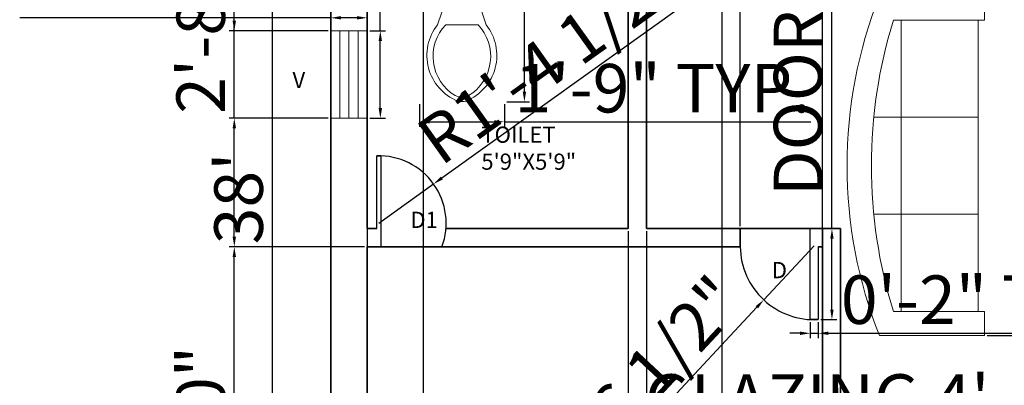
# Model space of a CAD drawing. Units: inches. Extents: x 2691 to 3133, y 1294 to 1993.
# Tile 2 of 7: x 2691 to 2935, y 1606 to 1696. Entities that reach past the tile are written whole.
import ezdxf

# ---------------------------------------------------------------- set-up
doc = ezdxf.new("R2010")
doc.units = ezdxf.units.IN
for name, color, linetype, lineweight in [('A-ANNO-DIMS', 2, 'Continuous', 18), ('A-ANNO-TEXT', 7, 'Continuous', 18), ('A-AREA-IDEN', 7, 'Continuous', 25), ('A-DOOR', 3, 'Continuous', 25), ('A-FLOR-FIXT', 9, 'Continuous', 18), ('A-FURN', 8, 'Continuous', 18), ('A-GLAZ', 4, 'Continuous', 18), ('A-WALL', 7, 'Continuous', 35)]:
    doc.layers.add(name, color=color, linetype=linetype, lineweight=lineweight)
doc.styles.get("Standard").update_dxf_attribs({"font": 'arial.ttf'})
doc.dimstyles.new('ISO-25', dxfattribs={"dimtxt": 12, "dimasz": 2.5, "dimexe": 1.25, "dimexo": 0.625, "dimtad": 1, "dimdec": 1, "dimlunit": 3, "dimtxsty": 'Standard', "dimcen": 2.5, "dimadec": 0, "dimazin": 0, "dimtfac": 1, "dimtdec": 1, "dimtmove": 0, "dimatfit": 3, "dimfxl": 1, "dimarcsym": 0})

# ---------------------------------------------------------------- blocks, each defined once
blk = doc.blocks.new('Sofa - Roundback 7 ft.')
for p, q in [((-12.00002, -32.4421), (-12.00003, -6.5971)), ((11.99997, -32.4421), (11.99998, -6.5971)), ((-36.000027, -34), (-36.000027, -11.4696)), ((35.99998, -34), (35.99998, -11.4696)), ((-35.999844, -13.3819), (35.9998, -13.3819)), ((-36.000027, -32.4421), (35.99998, -32.4421))]:
    blk.add_line(p, q)
for points in [[(-36.000027, -34), (-42.000027, -34), (-42.000027, -8)], [(41.99998, -8), (41.99998, -34), (35.99998, -34)]]:
    blk.add_lwpolyline(points)
for centre, radius, start, end in [((0, -114.25), 114.25, 68.43141, 111.5686), ((-0.00001, -127.1968), 121.1968, 72.72033, 107.2797)]:
    blk.add_arc(centre, radius, start, end)
blk = doc.blocks.new('Window - Wood Frame 36 in. Wide plan')
for p, q in [((0, 6), (0, 0)), ((36, 6), (36, 0)), ((0, 4.5), (36, 4.5)), ((0, 3), (36, 3)), ((0, 1.5), (36, 1.5))]:
    blk.add_line(p, q)
blk = doc.blocks.new('Toilet - top')
for p, q in [((9.5, -6), (9.5, -2)), ((-10, -8.5), (-8, -8.5)), ((-10, -9.5), (-10, -8.5)), ((-7, -9.5), (-10, -9.5)), ((-8, -8.5), (-8, -8)), ((-7, -8), (-7, -9.5)), ((-4, -8), (-6, -14)), ((4, -8), (6, -14)), ((4, -14), (-4, -14))]:
    blk.add_line(p, q)
blk.add_lwpolyline([(10.5, -8), (10.5, 0), (-10.5, 0), (-10.5, -8)], close=True)
for points in [[(-9.5, -2), (-9.5, -6)], [(8.5, -1), (-8.5, -1)], [(-8.5, -7), (8.5, -7)]]:
    blk.add_lwpolyline(points)
for centre, radius, start, end in [((-8.62, -1.88), 0.884, 81.8699, 188.1301), ((8.62, -1.88), 0.884, 351.8699, 98.1301), ((-8.62, -6.12), 0.884, 171.8699, 278.1301), ((8.62, -6.12), 0.884, 261.8699, 8.1301), ((3.52, -21.58), 12.17, 141.4691, 247.9714), ((4.2, -21.82), 11.33, 136.3677, 238.9468), ((-3.52, -21.58), 12.17, 292.0284, 38.5307), ((-4.2, -21.82), 11.33, 301.053, 43.6321), ((0, -27.88), 4, 245.7318, 294.2682), ((0, -29), 4, 254.8605, 285.1395)]:
    blk.add_arc(centre, radius, start, end)
blk = doc.blocks.new('*D11')
at = {"layer": 'A-ANNO-DIMS', "color": 0, "lineweight": -2, "transparency": 16777216}
for p, q in [((2767.62, 1880.05), (2752.52, 1880.05)), ((2753.77, 1877.55), (2753.77, 1426.55)), ((2767.62, 1424.05), (2752.52, 1424.05))]:
    blk.add_line(p, q, dxfattribs=at)
at = {"layer": 'A-ANNO-DIMS', "color": 0, "transparency": 16777216}
for points in [[(2753.35, 1877.55), (2754.18, 1877.55), (2753.77, 1880.05)], [(2753.35, 1426.55), (2754.18, 1426.55), (2753.77, 1424.05)]]:
    blk.add_solid(points, dxfattribs=at)
at = {"layer": 'Defpoints', "color": 0, "transparency": 16777216}
for p in [(2768.25, 1880.05), (2753.77, 1424.05), (2768.25, 1424.05)]:
    blk.add_point(p, dxfattribs=at)
at = {"layer": 'A-ANNO-DIMS', "color": 0, "transparency": 16777216, "insert": (2747.01, 1652.05), "char_height": 12, "attachment_point": 5, "rotation": 90}
blk.add_mtext("38'", dxfattribs=at)
blk = doc.blocks.new('DOOR-LEAF-THIN')
for p, q in [((18, 1), (0, 1)), ((0, 1), (0, 0)), ((0, 0), (22.5, 0))]:
    blk.add_line(p, q)
blk = doc.blocks.new('DOOR-LEAF-WIDE')
for p, q in [((0, 0), (0, 22.5)), ((2, 18), (2, 0)), ((2, 0), (0, 0))]:
    blk.add_line(p, q)
blk = doc.blocks.new('*D16')
at = {"layer": 'A-ANNO-DIMS', "color": 0, "lineweight": -2, "transparency": 16777216}
for p, q in [((2957.85, 1594.15), (2844.15, 1594.15)), ((2957.85, 1586.68), (2957.85, 1595.4)), ((3009.35, 1594.15), (2960.35, 1594.15)), ((3011.85, 1586.68), (3011.85, 1595.4))]:
    blk.add_line(p, q, dxfattribs=at)
at = {"layer": 'A-ANNO-DIMS', "color": 0, "transparency": 16777216}
for points in [[(2960.35, 1594.57), (2960.35, 1593.74), (2957.85, 1594.15)], [(3009.35, 1594.57), (3009.35, 1593.74), (3011.85, 1594.15)]]:
    blk.add_solid(points, dxfattribs=at)
at = {"layer": 'Defpoints', "color": 0, "transparency": 16777216}
for p in [(2957.85, 1594.15), (2957.85, 1586.05), (3011.85, 1586.05)]:
    blk.add_point(p, dxfattribs=at)
at = {"layer": 'A-ANNO-DIMS', "color": 0, "transparency": 16777216, "insert": (2899.75, 1600.98), "char_height": 12, "attachment_point": 5}
blk.add_mtext('GLAZING 4\'-6"', dxfattribs=at)
blk = doc.blocks.new('*D18')
at = {"layer": 'A-ANNO-DIMS', "color": 0, "lineweight": -2, "transparency": 16777216}
for p, q in [((2780.49, 1693.45), (2780.49, 1876.36)), ((2777.87, 1693.45), (2781.74, 1693.45)), ((2780.49, 1674.35), (2780.49, 1690.95)), ((2777.87, 1671.85), (2781.74, 1671.85))]:
    blk.add_line(p, q, dxfattribs=at)
at = {"layer": 'A-ANNO-DIMS', "color": 0, "transparency": 16777216}
for points in [[(2780.07, 1690.95), (2780.91, 1690.95), (2780.49, 1693.45)], [(2780.07, 1674.35), (2780.91, 1674.35), (2780.49, 1671.85)]]:
    blk.add_solid(points, dxfattribs=at)
at = {"layer": 'Defpoints', "color": 0, "transparency": 16777216}
for p in [(2777.25, 1693.45), (2780.49, 1693.45), (2777.25, 1671.85)]:
    blk.add_point(p, dxfattribs=at)
at = {"layer": 'A-ANNO-DIMS', "color": 0, "transparency": 16777216, "insert": (2773.66, 1786.16), "char_height": 12, "attachment_point": 5, "rotation": 90}
blk.add_mtext('GLAZING 1\'-9 1/2" TYP.', dxfattribs=at)
blk = doc.blocks.new('*D19')
at = {"layer": 'A-ANNO-DIMS', "color": 0, "lineweight": -2, "transparency": 16777216}
for p, q in [((2768.25, 1696.69), (2691.35, 1696.69)), ((2768.25, 1694.08), (2768.25, 1697.94)), ((2774.75, 1696.69), (2770.75, 1696.69)), ((2777.25, 1694.08), (2777.25, 1697.94))]:
    blk.add_line(p, q, dxfattribs=at)
at = {"layer": 'A-ANNO-DIMS', "color": 0, "transparency": 16777216}
for points in [[(2770.75, 1697.11), (2770.75, 1696.28), (2768.25, 1696.69)], [(2774.75, 1697.11), (2774.75, 1696.28), (2777.25, 1696.69)]]:
    blk.add_solid(points, dxfattribs=at)
at = {"layer": 'Defpoints', "color": 0, "transparency": 16777216}
for p in [(2768.25, 1696.69), (2768.25, 1693.45), (2777.25, 1693.45)]:
    blk.add_point(p, dxfattribs=at)
at = {"layer": 'A-ANNO-DIMS', "color": 0, "transparency": 16777216, "insert": (2728.55, 1703.44), "char_height": 12, "attachment_point": 5}
blk.add_mtext('0\'-9" TYP.', dxfattribs=at)
blk = doc.blocks.new('*D20')
at = {"layer": 'A-ANNO-DIMS', "color": 0, "lineweight": -2, "transparency": 16777216}
for p, q in [((2942.46, 1702.1), (2942.46, 1829.23)), ((2930.49, 1702.1), (2943.71, 1702.1)), ((2942.46, 1620.6), (2942.46, 1699.6)), ((2930.49, 1618.1), (2943.71, 1618.1))]:
    blk.add_line(p, q, dxfattribs=at)
at = {"layer": 'A-ANNO-DIMS', "color": 0, "transparency": 16777216}
for points in [[(2942.05, 1699.6), (2942.88, 1699.6), (2942.46, 1702.1)], [(2942.05, 1620.6), (2942.88, 1620.6), (2942.46, 1618.1)]]:
    blk.add_solid(points, dxfattribs=at)
at = {"layer": 'Defpoints', "color": 0, "transparency": 16777216}
for p in [(2929.86, 1702.1), (2942.46, 1702.1), (2929.86, 1618.1)]:
    blk.add_point(p, dxfattribs=at)
at = {"layer": 'A-ANNO-DIMS', "color": 0, "transparency": 16777216, "insert": (2935.63, 1766.91), "char_height": 12, "attachment_point": 5, "rotation": 90}
blk.add_mtext('SOFA 7\'-0" TYP.', dxfattribs=at)
blk = doc.blocks.new('*D21')
at = {"layer": 'A-ANNO-DIMS', "color": 0, "lineweight": -2, "transparency": 16777216}
for p, q in [((2893.2, 1702.72), (2893.2, 1715.95)), ((2929.86, 1702.72), (2929.86, 1715.95)), ((2893.2, 1714.7), (2788.35, 1714.7)), ((2927.36, 1714.7), (2895.7, 1714.7))]:
    blk.add_line(p, q, dxfattribs=at)
at = {"layer": 'A-ANNO-DIMS', "color": 0, "transparency": 16777216}
for points in [[(2895.7, 1715.11), (2895.7, 1714.28), (2893.2, 1714.7)], [(2927.36, 1715.11), (2927.36, 1714.28), (2929.86, 1714.7)]]:
    blk.add_solid(points, dxfattribs=at)
at = {"layer": 'Defpoints', "color": 0, "transparency": 16777216}
for p in [(2893.2, 1714.7), (2893.2, 1702.1), (2929.86, 1702.1)]:
    blk.add_point(p, dxfattribs=at)
at = {"layer": 'A-ANNO-DIMS', "color": 0, "transparency": 16777216, "insert": (2839.52, 1721.53), "char_height": 12, "attachment_point": 5}
blk.add_mtext('3\'-0 1/2" TYP.', dxfattribs=at)
blk = doc.blocks.new('*D22')
at = {"layer": 'A-ANNO-DIMS', "color": 0, "lineweight": -2, "transparency": 16777216}
for p, q in [((2816.11, 1708.98), (2816.11, 1818.95)), ((2811.78, 1708.98), (2817.36, 1708.98)), ((2816.11, 1678.43), (2816.11, 1706.48)), ((2811.78, 1675.93), (2817.36, 1675.93))]:
    blk.add_line(p, q, dxfattribs=at)
at = {"layer": 'A-ANNO-DIMS', "color": 0, "transparency": 16777216}
for points in [[(2815.69, 1706.48), (2816.52, 1706.48), (2816.11, 1708.98)], [(2815.69, 1678.43), (2816.52, 1678.43), (2816.11, 1675.93)]]:
    blk.add_solid(points, dxfattribs=at)
at = {"layer": 'Defpoints', "color": 0, "transparency": 16777216}
for p in [(2811.15, 1708.98), (2816.11, 1708.98), (2811.15, 1675.93)]:
    blk.add_point(p, dxfattribs=at)
at = {"layer": 'A-ANNO-DIMS', "color": 0, "transparency": 16777216, "insert": (2809.28, 1765.22), "char_height": 12, "attachment_point": 5, "rotation": 90}
blk.add_mtext('WC 2\'-9" TYP.', dxfattribs=at)
blk = doc.blocks.new('*D23')
at = {"layer": 'A-ANNO-DIMS', "color": 0, "lineweight": -2, "transparency": 16777216}
for p, q in [((2790.15, 1675.31), (2790.15, 1669.73)), ((2811.15, 1675.31), (2811.15, 1669.73)), ((2792.65, 1670.98), (2808.65, 1670.98)), ((2811.15, 1670.98), (2886.92, 1670.98))]:
    blk.add_line(p, q, dxfattribs=at)
at = {"layer": 'A-ANNO-DIMS', "color": 0, "transparency": 16777216}
for points in [[(2792.65, 1671.39), (2792.65, 1670.56), (2790.15, 1670.98)], [(2808.65, 1671.39), (2808.65, 1670.56), (2811.15, 1670.98)]]:
    blk.add_solid(points, dxfattribs=at)
at = {"layer": 'Defpoints', "color": 0, "transparency": 16777216}
for p in [(2790.15, 1675.93), (2811.15, 1675.93), (2811.15, 1670.98)]:
    blk.add_point(p, dxfattribs=at)
at = {"layer": 'A-ANNO-DIMS', "color": 0, "transparency": 16777216, "insert": (2850.28, 1677.73), "char_height": 12, "attachment_point": 5}
blk.add_mtext('1\'-9" TYP.', dxfattribs=at)
blk = doc.blocks.new('*D26')
at = {"layer": 'A-ANNO-DIMS', "color": 0, "lineweight": -2, "transparency": 16777216}
for p, q in [((2892.12, 1644.55), (2892.12, 1859.67)), ((2889.37, 1644.55), (2893.37, 1644.55)), ((2892.12, 1624.55), (2892.12, 1642.05)), ((2889.37, 1622.05), (2893.37, 1622.05))]:
    blk.add_line(p, q, dxfattribs=at)
at = {"layer": 'A-ANNO-DIMS', "color": 0, "transparency": 16777216}
for points in [[(2891.71, 1642.05), (2892.54, 1642.05), (2892.12, 1644.55)], [(2891.71, 1624.55), (2892.54, 1624.55), (2892.12, 1622.05)]]:
    blk.add_solid(points, dxfattribs=at)
at = {"layer": 'Defpoints', "color": 0, "transparency": 16777216}
for p in [(2888.75, 1644.55), (2892.12, 1644.55), (2888.75, 1622.05)]:
    blk.add_point(p, dxfattribs=at)
at = {"layer": 'A-ANNO-DIMS', "color": 0, "transparency": 16777216, "insert": (2885.29, 1753.36), "char_height": 12, "attachment_point": 5, "rotation": 90}
blk.add_mtext('DOOR LEAF 1\'-10 1/2" TYP.', dxfattribs=at)
blk = doc.blocks.new('*D27')
at = {"layer": 'A-ANNO-DIMS', "color": 0, "lineweight": -2, "transparency": 16777216}
for p, q in [((2886.75, 1621.43), (2886.75, 1617.43)), ((2888.75, 1621.43), (2888.75, 1617.43)), ((2884.25, 1618.68), (2881.75, 1618.68)), ((2886.75, 1618.68), (2888.75, 1618.68)), ((2891.25, 1618.68), (2968.15, 1618.68))]:
    blk.add_line(p, q, dxfattribs=at)
at = {"layer": 'A-ANNO-DIMS', "color": 0, "transparency": 16777216}
for points in [[(2884.25, 1619.1), (2884.25, 1618.26), (2886.75, 1618.68)], [(2891.25, 1619.1), (2891.25, 1618.26), (2888.75, 1618.68)]]:
    blk.add_solid(points, dxfattribs=at)
at = {"layer": 'Defpoints', "color": 0, "transparency": 16777216}
for p in [(2886.75, 1622.05), (2888.75, 1622.05), (2888.75, 1618.68)]:
    blk.add_point(p, dxfattribs=at)
at = {"layer": 'A-ANNO-DIMS', "color": 0, "transparency": 16777216, "insert": (2930.95, 1625.43), "char_height": 12, "attachment_point": 5}
blk.add_mtext('0\'-2" TYP.', dxfattribs=at)
blk = doc.blocks.new('*D44')
at = {"layer": 'A-ANNO-DIMS', "color": 0, "lineweight": -2, "transparency": 16777216}
for p, q in [((2776.62, 1640.05), (2743.15, 1640.05)), ((2744.4, 1548.33), (2744.4, 1637.55)), ((2767.62, 1545.83), (2743.15, 1545.83))]:
    blk.add_line(p, q, dxfattribs=at)
at = {"layer": 'A-ANNO-DIMS', "color": 0, "transparency": 16777216}
for points in [[(2743.98, 1637.55), (2744.82, 1637.55), (2744.4, 1640.05)], [(2743.98, 1548.33), (2744.82, 1548.33), (2744.4, 1545.83)]]:
    blk.add_solid(points, dxfattribs=at)
at = {"layer": 'Defpoints', "color": 0, "transparency": 16777216}
for p in [(2744.4, 1640.05), (2777.25, 1640.05), (2768.25, 1545.83)]:
    blk.add_point(p, dxfattribs=at)
at = {"layer": 'A-ANNO-DIMS', "color": 0, "transparency": 16777216, "insert": (2737.65, 1592.94), "char_height": 12, "attachment_point": 5, "rotation": 90}
blk.add_mtext('7\'-10"', dxfattribs=at)
blk = doc.blocks.new('*D45')
at = {"layer": 'A-ANNO-DIMS', "color": 0, "lineweight": -2, "transparency": 16777216}
for p, q in [((2744.4, 1671.85), (2744.4, 1707.71)), ((2767.62, 1671.85), (2743.15, 1671.85)), ((2744.4, 1642.55), (2744.4, 1669.35)), ((2776.62, 1640.05), (2743.15, 1640.05))]:
    blk.add_line(p, q, dxfattribs=at)
at = {"layer": 'A-ANNO-DIMS', "color": 0, "transparency": 16777216}
for points in [[(2743.98, 1669.35), (2744.82, 1669.35), (2744.4, 1671.85)], [(2743.98, 1642.55), (2744.82, 1642.55), (2744.4, 1640.05)]]:
    blk.add_solid(points, dxfattribs=at)
at = {"layer": 'Defpoints', "color": 0, "transparency": 16777216}
for p in [(2744.4, 1671.85), (2768.25, 1671.85), (2777.25, 1640.05)]:
    blk.add_point(p, dxfattribs=at)
at = {"layer": 'A-ANNO-DIMS', "color": 0, "transparency": 16777216, "insert": (2737.65, 1691.03), "char_height": 12, "attachment_point": 5, "rotation": 90}
blk.add_mtext('2\'-8"', dxfattribs=at)
blk = doc.blocks.new('*D46')
at = {"layer": 'A-ANNO-DIMS', "color": 0, "lineweight": -2, "transparency": 16777216}
for p, q in [((2744.4, 1720.1), (2744.4, 1783.91)), ((2767.62, 1720.1), (2743.15, 1720.1)), ((2744.4, 1695.95), (2744.4, 1717.6)), ((2767.62, 1693.45), (2743.15, 1693.45))]:
    blk.add_line(p, q, dxfattribs=at)
at = {"layer": 'A-ANNO-DIMS', "color": 0, "transparency": 16777216}
for points in [[(2743.98, 1717.6), (2744.82, 1717.6), (2744.4, 1720.1)], [(2743.98, 1695.95), (2744.82, 1695.95), (2744.4, 1693.45)]]:
    blk.add_solid(points, dxfattribs=at)
at = {"layer": 'Defpoints', "color": 0, "transparency": 16777216}
for p in [(2744.4, 1720.1), (2768.25, 1720.1), (2768.25, 1693.45)]:
    blk.add_point(p, dxfattribs=at)
at = {"layer": 'A-ANNO-DIMS', "color": 0, "transparency": 16777216, "insert": (2737.57, 1753.25), "char_height": 12, "attachment_point": 5, "rotation": 90}
blk.add_mtext('2\'-2 1/2"', dxfattribs=at)
blk = doc.blocks.new('*D54')
at = {"layer": 'A-ANNO-DIMS', "color": 0, "lineweight": -2, "transparency": 16777216}
for p, q in [((2846.25, 1645.18), (2846.25, 1905.15)), ((2848.75, 1903.9), (2866.94, 1903.9)), ((2869.44, 1645.18), (2869.44, 1905.15)), ((2869.44, 1903.9), (2913.28, 1903.9))]:
    blk.add_line(p, q, dxfattribs=at)
at = {"layer": 'A-ANNO-DIMS', "color": 0, "transparency": 16777216}
for points in [[(2848.75, 1904.32), (2848.75, 1903.49), (2846.25, 1903.9)], [(2866.94, 1904.32), (2866.94, 1903.49), (2869.44, 1903.9)]]:
    blk.add_solid(points, dxfattribs=at)
at = {"layer": 'Defpoints', "color": 0, "transparency": 16777216}
for p in [(2869.44, 1903.9), (2846.25, 1644.55), (2869.44, 1644.55)]:
    blk.add_point(p, dxfattribs=at)
at = {"layer": 'A-ANNO-DIMS', "color": 0, "transparency": 16777216, "insert": (2892.61, 1910.55), "char_height": 12, "attachment_point": 5}
blk.add_mtext('1\'-11"', dxfattribs=at)
blk = doc.blocks.new('*D55')
at = {"layer": 'A-ANNO-DIMS', "color": 0, "lineweight": -2, "transparency": 16777216}
for p, q in [((2841.75, 1643.93), (2841.75, 1398.95)), ((2846.25, 1643.93), (2846.25, 1398.95)), ((2839.25, 1400.2), (2836.75, 1400.2)), ((2841.75, 1400.2), (2846.25, 1400.2)), ((2848.75, 1400.2), (2912.36, 1400.2))]:
    blk.add_line(p, q, dxfattribs=at)
at = {"layer": 'A-ANNO-DIMS', "color": 0, "transparency": 16777216}
for points in [[(2839.25, 1400.62), (2839.25, 1399.79), (2841.75, 1400.2)], [(2848.75, 1400.62), (2848.75, 1399.79), (2846.25, 1400.2)]]:
    blk.add_solid(points, dxfattribs=at)
at = {"layer": 'Defpoints', "color": 0, "transparency": 16777216}
for p in [(2841.75, 1644.55), (2846.25, 1644.55), (2846.25, 1400.2)]:
    blk.add_point(p, dxfattribs=at)
at = {"layer": 'A-ANNO-DIMS', "color": 0, "transparency": 16777216, "insert": (2881.8, 1407.03), "char_height": 12, "attachment_point": 5}
blk.add_mtext('0\'-4 1/2"', dxfattribs=at)
blk = doc.blocks.new('*D56')
at = {"layer": 'A-ANNO-DIMS', "color": 0, "lineweight": -2, "transparency": 16777216}
for p, q in [((2846.25, 1643.93), (2846.25, 1398.95)), ((2777.25, 1639.43), (2777.25, 1398.95)), ((2779.75, 1400.2), (2843.75, 1400.2))]:
    blk.add_line(p, q, dxfattribs=at)
at = {"layer": 'A-ANNO-DIMS', "color": 0, "transparency": 16777216}
for points in [[(2779.75, 1400.62), (2779.75, 1399.79), (2777.25, 1400.2)], [(2843.75, 1400.62), (2843.75, 1399.79), (2846.25, 1400.2)]]:
    blk.add_solid(points, dxfattribs=at)
at = {"layer": 'Defpoints', "color": 0, "transparency": 16777216}
for p in [(2846.25, 1644.55), (2777.25, 1640.05), (2846.25, 1400.2)]:
    blk.add_point(p, dxfattribs=at)
at = {"layer": 'A-ANNO-DIMS', "color": 0, "transparency": 16777216, "insert": (2811.75, 1406.96), "char_height": 12, "attachment_point": 5}
blk.add_mtext('5\'-9"', dxfattribs=at)
blk = doc.blocks.new('*D58')
at = {"layer": 'A-ANNO-DIMS', "color": 0, "lineweight": -2, "transparency": 16777216}
for p, q in [((2777.25, 1756.43), (2777.25, 1398.95)), ((2791.1, 1756.43), (2791.1, 1398.95)), ((2779.75, 1400.2), (2788.6, 1400.2)), ((2791.1, 1400.2), (2825.62, 1400.2))]:
    blk.add_line(p, q, dxfattribs=at)
at = {"layer": 'A-ANNO-DIMS', "color": 0, "transparency": 16777216}
for points in [[(2779.75, 1400.62), (2779.75, 1399.79), (2777.25, 1400.2)], [(2788.6, 1400.62), (2788.6, 1399.79), (2791.1, 1400.2)]]:
    blk.add_solid(points, dxfattribs=at)
at = {"layer": 'Defpoints', "color": 0, "transparency": 16777216}
for p in [(2777.25, 1757.05), (2791.1, 1757.05), (2791.1, 1400.2)]:
    blk.add_point(p, dxfattribs=at)
at = {"layer": 'A-ANNO-DIMS', "color": 0, "transparency": 16777216, "insert": (2809.61, 1406.85), "char_height": 12, "attachment_point": 5}
blk.add_mtext('1\'-2"', dxfattribs=at)
blk = doc.blocks.new('*D61')
at = {"layer": 'A-ANNO-DIMS', "color": 0, "lineweight": -2, "transparency": 16777216}
for p, q in [((2864.96, 1433.88), (2864.96, 1905.15)), ((2867.46, 1903.9), (2887.25, 1903.9)), ((2889.75, 1433.68), (2889.75, 1905.15)), ((2889.75, 1903.9), (2925.6, 1903.9))]:
    blk.add_line(p, q, dxfattribs=at)
at = {"layer": 'A-ANNO-DIMS', "color": 0, "transparency": 16777216}
for points in [[(2867.46, 1904.32), (2867.46, 1903.49), (2864.96, 1903.9)], [(2887.25, 1904.32), (2887.25, 1903.49), (2889.75, 1903.9)]]:
    blk.add_solid(points, dxfattribs=at)
at = {"layer": 'Defpoints', "color": 0, "transparency": 16777216}
for p in [(2889.75, 1903.9), (2864.96, 1433.26), (2889.75, 1433.05)]:
    blk.add_point(p, dxfattribs=at)
at = {"layer": 'A-ANNO-DIMS', "color": 0, "transparency": 16777216, "insert": (2908.93, 1910.55), "char_height": 12, "attachment_point": 5}
blk.add_mtext('2\'-1"', dxfattribs=at)
blk = doc.blocks.new('*D63')
at = {"layer": 'A-ANNO-DIMS', "color": 0, "lineweight": -2, "transparency": 16777216}
for p, q in [((2887.75, 1640.32), (2875.27, 1626.95)), ((2822.33, 1570.22), (2873.57, 1625.12))]:
    blk.add_line(p, q, dxfattribs=at)
at = {"layer": 'A-ANNO-DIMS', "color": 0, "transparency": 16777216}
blk.add_solid([(2873.26, 1625.4), (2873.87, 1624.83), (2875.27, 1626.95)], dxfattribs=at)
at = {"layer": 'Defpoints', "color": 0, "transparency": 16777216}
for p in [(2887.75, 1640.32), (2875.27, 1626.95)]:
    blk.add_point(p, dxfattribs=at)
at = {"layer": 'A-ANNO-DIMS', "color": 0, "transparency": 16777216, "insert": (2842.1, 1601.41), "char_height": 12, "attachment_point": 5, "rotation": 46.9754}
blk.add_mtext('R1\'-6 1/2"', dxfattribs=at)
blk = doc.blocks.new('*D64')
at = {"layer": 'A-ANNO-DIMS', "color": 0, "lineweight": -2, "transparency": 16777216}
for p, q in [((2856.77, 1700.76), (2795.71, 1657.05)), ((2780.12, 1645.9), (2793.67, 1655.6))]:
    blk.add_line(p, q, dxfattribs=at)
at = {"layer": 'A-ANNO-DIMS', "color": 0, "transparency": 16777216}
blk.add_solid([(2795.46, 1657.39), (2795.95, 1656.71), (2793.67, 1655.6)], dxfattribs=at)
at = {"layer": 'Defpoints', "color": 0, "transparency": 16777216}
for p in [(2793.67, 1655.6), (2780.12, 1645.9)]:
    blk.add_point(p, dxfattribs=at)
at = {"layer": 'A-ANNO-DIMS', "color": 0, "transparency": 16777216, "insert": (2823.28, 1685.19), "char_height": 12, "attachment_point": 5, "rotation": 35.5904}
blk.add_mtext('R1\'-4 1/2"', dxfattribs=at)

msp = doc.modelspace()

# ---------------------------------------------------------------- linework, layer by layer
at = {"layer": 'A-DOOR'}
for centre, radius, start, end in [((2780.12, 1645.9), 16.66, 339.4601, 91.7197), ((2887.75, 1640.32), 18.29, 180.8182, 273.1344)]:
    msp.add_arc(centre, radius, start, end, dxfattribs=at)
at = {"layer": 'A-WALL'}
for p, q in [((2768.25, 1880.05), (2768.25, 1424.05)), ((2777.25, 1757.05), (2777.25, 1644.55)), ((2846.25, 1757.05), (2846.25, 1644.55)), ((2841.75, 1709.05), (2841.75, 1644.55)), ((2779.62, 1644.55), (2777.25, 1644.55)), ((2841.75, 1644.55), (2796.73, 1644.55)), ((2894.25, 1644.55), (2846.25, 1644.55)), ((2886.75, 1644.55), (2859.52, 1644.55)), ((2869.44, 1644.55), (2869.44, 1640.05)), ((2886.75, 1644.55), (2886.75, 1644.55)), ((2889.75, 1644.55), (2888.75, 1644.55)), ((2889.75, 1644.55), (2889.75, 1433.05)), ((2894.25, 1644.55), (2894.25, 1424.05)), ((2777.25, 1640.05), (2777.25, 1433.05)), ((2869.46, 1640.05), (2777.25, 1640.05)), ((2780.62, 1640.05), (2795.73, 1640.05)), ((2889.75, 1640.05), (2888.75, 1640.05))]:
    msp.add_line(p, q, dxfattribs=at)

# ---------------------------------------------------------------- block references
at = {"layer": 'A-DOOR', "extrusion": (0, 0, -1), "zscale": -1, "rotation": 270}
msp.add_blockref('DOOR-LEAF-THIN', (-2780.62, 1662.55), dxfattribs=at)
at = {"layer": 'A-DOOR'}
msp.add_blockref('DOOR-LEAF-WIDE', (2886.75, 1622.05), dxfattribs=at)
at = {"layer": 'A-FLOR-FIXT'}
msp.add_blockref('Toilet - top', (2800.65, 1708.98), dxfattribs=at)
at = {"layer": 'A-FURN', "rotation": 90}
msp.add_blockref('Sofa - Roundback 7 ft.', (2895.86, 1660.1), dxfattribs=at)
at = {"layer": 'A-GLAZ', "xscale": 0.6, "yscale": 1.5, "rotation": 90}
msp.add_blockref('Window - Wood Frame 36 in. Wide plan', (2777.25, 1671.85), dxfattribs=at)

# ---------------------------------------------------------------- texts
at = {"layer": 'A-ANNO-TEXT', "char_height": 4, "attachment_point": 1}
for s, insert in [('V', (2758.78, 1683.3)), ('D1', (2787.92, 1648.73)), ('D', (2877.26, 1636.3))]:
    msp.add_mtext_dynamic_manual_height_columns(s, width=0.1038, gutter_width=12.5, heights=[0], dxfattribs=dict(at, insert=insert))
at = {"layer": 'A-AREA-IDEN', "insert": (2805.46, 1669.79), "char_height": 4, "attachment_point": 1}
msp.add_mtext_dynamic_manual_height_columns('TOILET\\P5\'9"X5\'9"', width=1.3496, gutter_width=12.5, heights=[0], dxfattribs=at)

# ---------------------------------------------------------------- dimensions: what is measured, and where the dimension line sits
at = {"layer": 'A-ANNO-DIMS'}
for base, p1, p2, picture, middle in [((2869.44, 1903.9), (2846.25, 1644.55), (2869.44, 1644.55), '*D54', (2892.61, 1910.55)), ((2889.75, 1903.9), (2864.96, 1433.26), (2889.75, 1433.05), '*D61', (2908.93, 1910.55)), ((2791.0965, 1400.2049), (2777.2496, 1757.0549), (2791.0965, 1757.0549), '*D58', (2809.6063, 1406.8545)), ((2846.25, 1400.2), (2777.25, 1640.05), (2846.25, 1644.55), '*D56', (2811.75, 1406.96)), ((2846.25, 1400.2), (2841.75, 1644.55), (2846.25, 1644.55), '*D55', (2881.8, 1407.03))]:
    dim = msp.add_linear_dim(base=base, p1=p1, p2=p2, dimstyle='ISO-25', override={"dimdec": 1, "dimlfac": 1, "dimrnd": 0, "dimzin": 1, "dimdsep": 46, "dimlunit": 4, "dimfrac": 2}, dxfattribs=at)
    dim.commit()
    dim.dimension.update_dxf_attribs({"geometry": picture, "text_midpoint": middle})
for base, p1, p2, override, picture, middle in [((2753.77, 1424.05), (2768.25, 1880.05), (2768.25, 1424.05), {"dimclrd": 0, "dimclre": 0, "dimclrt": 0}, '*D11', (2747.01, 1652.05)), ((2744.3996, 1720.0971), (2768.2496, 1693.4519), (2768.2496, 1720.0971), {"dimdec": 1, "dimlfac": 1, "dimrnd": 0, "dimzin": 1, "dimdsep": 46, "dimlunit": 4, "dimfrac": 2}, '*D46', (2737.5699, 1753.2548)), ((2744.4, 1671.85), (2777.25, 1640.05), (2768.25, 1671.85), {"dimdec": 1, "dimlfac": 1, "dimrnd": 0, "dimzin": 1, "dimdsep": 46, "dimlunit": 4, "dimfrac": 2}, '*D45', (2737.65, 1691.03)), ((2744.4, 1640.05), (2768.25, 1545.83), (2777.25, 1640.05), {"dimdec": 1, "dimlfac": 1, "dimrnd": 0, "dimzin": 1, "dimdsep": 46, "dimlunit": 4, "dimfrac": 2}, '*D44', (2737.65, 1592.94))]:
    dim = msp.add_linear_dim(base=base, p1=p1, p2=p2, angle=90, dimstyle='ISO-25', override=override, dxfattribs=at)
    dim.commit()
    dim.dimension.update_dxf_attribs({"geometry": picture, "text_midpoint": middle})
for base, p1, p2, angle, text, picture, middle in [((2780.49, 1693.45), (2777.25, 1671.85), (2777.25, 1693.45), 90, 'GLAZING <> TYP.', '*D18', (2773.66, 1786.16)), ((2892.12, 1644.55), (2888.75, 1622.05), (2888.75, 1644.55), 90, 'DOOR LEAF <> TYP.', '*D26', (2885.29, 1753.36)), ((2942.46, 1702.1), (2929.86, 1618.1), (2929.86, 1702.1), 90, 'SOFA <> TYP.', '*D20', (2935.63, 1766.91)), ((2816.1072, 1708.9801), (2811.1502, 1675.9339), (2811.1502, 1708.9801), 90, 'WC <> TYP.', '*D22', (2809.2775, 1765.217)), ((2893.2, 1714.7), (2929.86, 1702.1), (2893.2, 1702.1), 180, '<> TYP.', '*D21', (2839.52, 1721.53)), ((2768.25, 1696.69), (2777.25, 1693.45), (2768.25, 1693.45), 180, '<> TYP.', '*D19', (2728.55, 1703.44)), ((2957.85, 1594.15), (3011.85, 1586.05), (2957.85, 1586.05), 180, 'GLAZING <>', '*D16', (2899.75, 1600.98))]:
    dim = msp.add_linear_dim(base=base, p1=p1, p2=p2, angle=angle, text=text, dimstyle='ISO-25', override={"dimdec": 1, "dimlfac": 1, "dimrnd": 0, "dimzin": 1, "dimdsep": 46, "dimlunit": 4, "dimfrac": 2}, dxfattribs=at)
    dim.commit()
    dim.dimension.update_dxf_attribs({"geometry": picture, "text_midpoint": middle})
for center, mpoint, picture, middle in [((2780.12, 1645.9), (2793.67, 1655.6), '*D64', (2823.28, 1685.19)), ((2887.75, 1640.32), (2875.27, 1626.95), '*D63', (2842.1, 1601.41))]:
    dim = msp.add_radius_dim(center=center, mpoint=mpoint, dimstyle='ISO-25', override={"dimdec": 1, "dimlfac": 1, "dimrnd": 0, "dimzin": 1, "dimdsep": 46, "dimlunit": 4, "dimfrac": 2}, dxfattribs=at)
    dim.commit()
    dim.dimension.update_dxf_attribs({"geometry": picture, "text_midpoint": middle})
for base, p1, p2, picture, middle in [((2811.15, 1670.98), (2790.15, 1675.93), (2811.15, 1675.93), '*D23', (2850.28, 1677.73)), ((2888.75, 1618.68), (2886.75, 1622.05), (2888.75, 1622.05), '*D27', (2930.95, 1625.43))]:
    dim = msp.add_linear_dim(base=base, p1=p1, p2=p2, text='<> TYP.', dimstyle='ISO-25', override={"dimdec": 1, "dimlfac": 1, "dimrnd": 0, "dimzin": 1, "dimdsep": 46, "dimlunit": 4, "dimfrac": 2}, dxfattribs=at)
    dim.commit()
    dim.dimension.update_dxf_attribs({"geometry": picture, "text_midpoint": middle})

doc.saveas('drawing.dxf')
